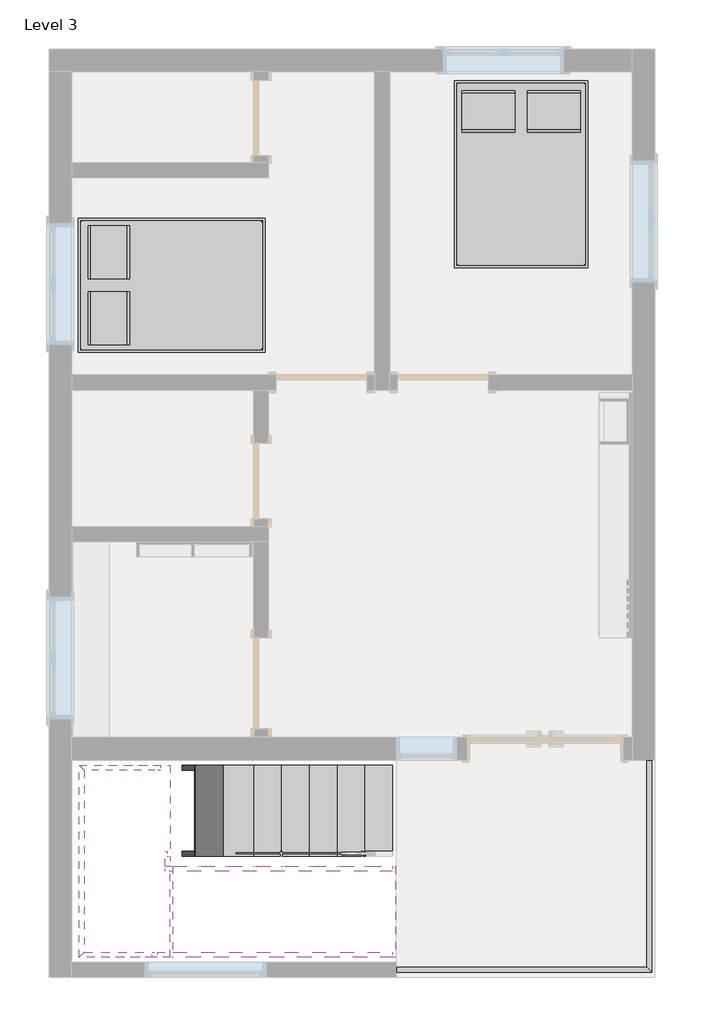
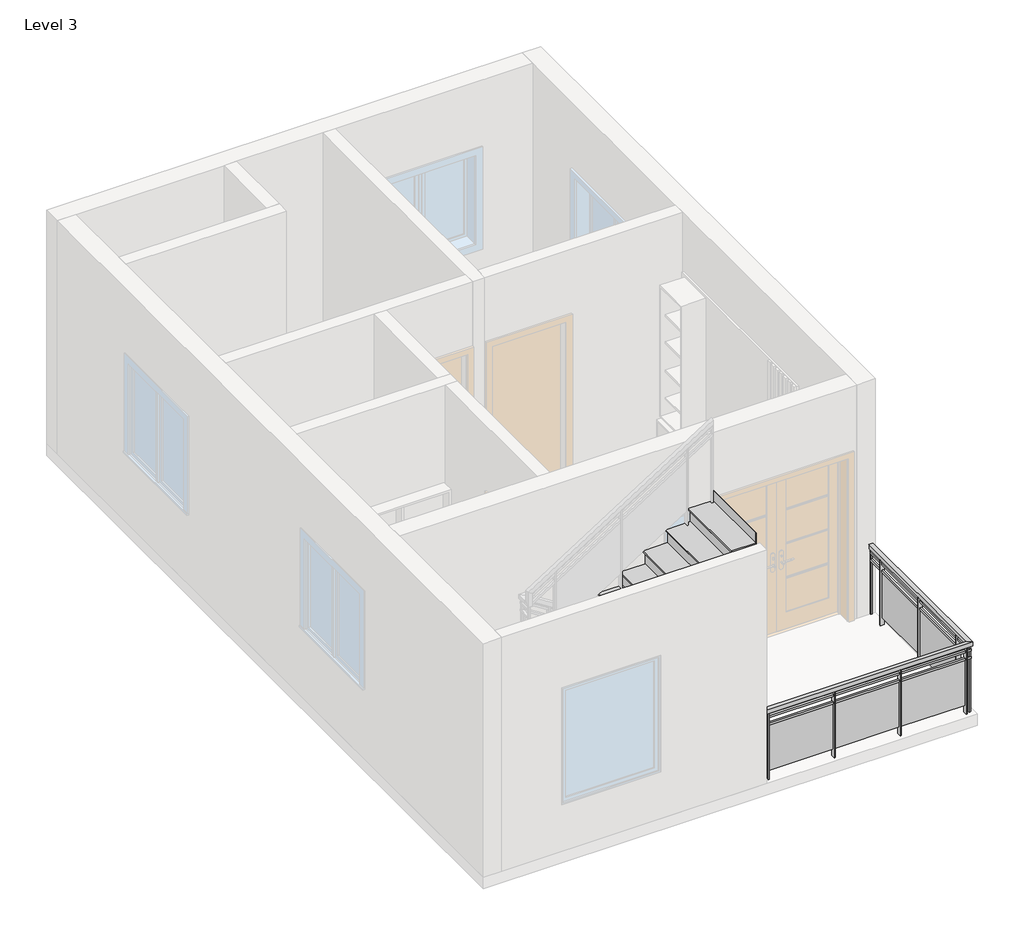
# One storey, part 2 of 2: 8 members, 2 furniture elements, 2 stair flights, 1 railing, 1 slab.
"""IFC4 building model written with IfcOpenShell, lengths in millimetres."""

from ifc_helpers import new_model, si_unit, frame, origin, place, context, project, spatial, polyline, outline, extrude, faceted_brep, transform, mapped, element, save
from components import furniture_c8abb964, non_monolithic_landing_73a33424, stair_flight_79624163, stair_flight_1f3fe34f

model = new_model("IFC4")

# Units and contexts
model_context = context("Model", 3, world=origin())
ifc_project = project(units=[si_unit("LENGTHUNIT", "METRE", prefix="MILLI")], contexts=[model_context])

# Site, building, storey
site = spatial("IfcSite", under=ifc_project)
building = spatial("IfcBuilding", under=site)
storey = spatial("IfcBuildingStorey", under=building, Name="Level 3", Elevation=6400.8)

# Furniture
placement = place(None, origin())
furniture_shape = furniture_c8abb964(model_context)
element("IfcFurniture", 1, ObjectType="Bed-Box : Double 53\" x 74\"", at=placement, inside=storey, context=model_context, shape_type="MappedRepresentation", body=[
    mapped(furniture_shape, transform((-5702.2407796, -383.210135, 6400.8), x_axis=(0.0, 0.9999999999999999, 0.0), y_axis=(-0.9999999999999999, 0.0, 0.0), z_axis=(0.0, 0.0, 1.0))),
])
element("IfcFurniture", 2, ObjectType="Bed-Box : Double 53\" x 74\"", at=placement, inside=storey, context=model_context, shape_type="MappedRepresentation", body=[
    mapped(furniture_shape, transform((-2289.0637304, 1307.9718322, 6400.8), x_axis=(1.0, 0.0, 0.0), y_axis=(0.0, 1.0, 0.0), z_axis=(0.0, 0.0, 1.0))),
])

# Members
element("IfcMember", 3, ObjectType="Carriage - 2\" Width", at=placement, inside=storey, context=model_context, shape_type="Brep", body=[
    faceted_brep([(-3245.3112714, -5936.857676, 9277.1282995), (-3245.3112714, -5886.057676, 9277.1282995), (-3245.3112714, -5886.057676, 9372.6), (-3245.3112714, -5936.857676, 9372.6), (-3492.9612714, -5886.057676, 9119.532845), (-3772.3612714, -5886.057676, 8941.732845), (-4051.7612714, -5886.057676, 8763.932845), (-4331.1612714, -5886.057676, 8586.132845), (-4610.5612714, -5886.057676, 8408.332845), (-4889.9612714, -5886.057676, 8230.532845), (-5169.3612714, -5886.057676, 8052.732845), (-5448.7612714, -5886.057676, 7874.932845), (-5480.5112714, -5886.057676, 7854.7282995), (-5531.3112714, -5886.057676, 7822.4010268), (-5531.3112714, -5886.057676, 7950.2), (-5480.5112714, -5886.057676, 7950.2), (-5448.7612714, -5886.057676, 7950.2), (-5448.7612714, -5886.057676, 8128.0), (-5169.3612714, -5886.057676, 8128.0), (-5169.3612714, -5886.057676, 8305.8), (-4889.9612714, -5886.057676, 8305.8), (-4889.9612714, -5886.057676, 8483.6), (-4610.5612714, -5886.057676, 8483.6), (-4610.5612714, -5886.057676, 8661.4), (-4331.1612714, -5886.057676, 8661.4), (-4331.1612714, -5886.057676, 8839.2), (-4051.7612714, -5886.057676, 8839.2), (-4051.7612714, -5886.057676, 9017.0), (-3772.3612714, -5886.057676, 9017.0), (-3772.3612714, -5886.057676, 9194.8), (-3492.9612714, -5886.057676, 9194.8), (-3492.9612714, -5886.057676, 9372.6), (-5531.3112714, -5936.857676, 7822.4010268), (-3492.9612714, -5936.857676, 9372.6), (-3492.9612714, -5936.857676, 9194.8), (-3772.3612714, -5936.857676, 9194.8), (-3772.3612714, -5936.857676, 9017.0), (-4051.7612714, -5936.857676, 9017.0), (-4051.7612714, -5936.857676, 8839.2), (-4331.1612714, -5936.857676, 8839.2), (-4331.1612714, -5936.857676, 8661.4), (-4610.5612714, -5936.857676, 8661.4), (-4610.5612714, -5936.857676, 8483.6), (-4889.9612714, -5936.857676, 8483.6), (-4889.9612714, -5936.857676, 8305.8), (-5169.3612714, -5936.857676, 8305.8), (-5169.3612714, -5936.857676, 8128.0), (-5448.7612714, -5936.857676, 8128.0), (-5448.7612714, -5936.857676, 7950.2), (-5531.3112714, -5936.857676, 7950.2)], [[[0, 1, 2, 3]], [[2, 1, 4, 5, 6, 7, 8, 9, 10, 11, 12, 13, 14, 15, 16, 17, 18, 19, 20, 21, 22, 23, 24, 25, 26, 27, 28, 29, 30, 31]], [[1, 0, 32, 13, 12, 11, 10, 9, 8, 7, 6, 5, 4]], [[32, 0, 3, 33, 34, 35, 36, 37, 38, 39, 40, 41, 42, 43, 44, 45, 46, 47, 48, 49]], [[17, 47, 46, 18]], [[47, 17, 16, 48]], [[19, 45, 44, 20]], [[18, 46, 45, 19]], [[21, 43, 42, 22]], [[20, 44, 43, 21]], [[23, 41, 40, 24]], [[22, 42, 41, 23]], [[25, 39, 38, 26]], [[24, 40, 39, 25]], [[27, 37, 36, 28]], [[26, 38, 37, 27]], [[29, 35, 34, 30]], [[28, 36, 35, 29]], [[31, 33, 3, 2]], [[30, 34, 33, 31]], [[13, 32, 49, 14]], [[48, 16, 15, 14, 49]]]),
])
element("IfcMember", 4, ObjectType="Carriage - 2\" Width", at=placement, inside=storey, context=model_context, shape_type="Brep", body=[
    faceted_brep([(-3245.3112714, -6800.457676, 9277.1282995), (-3245.3112714, -6749.657676, 9277.1282995), (-3245.3112714, -6749.657676, 9372.6), (-3245.3112714, -6800.457676, 9372.6), (-5609.8843135, -6749.657676, 7772.4), (-5661.6597957, -6749.657676, 7950.2), (-5448.7612714, -6749.657676, 7950.2), (-5448.7612714, -6749.657676, 8128.0), (-5169.3612714, -6749.657676, 8128.0), (-5169.3612714, -6749.657676, 8305.8), (-4889.9612714, -6749.657676, 8305.8), (-4889.9612714, -6749.657676, 8483.6), (-4610.5612714, -6749.657676, 8483.6), (-4610.5612714, -6749.657676, 8661.4), (-4331.1612714, -6749.657676, 8661.4), (-4331.1612714, -6749.657676, 8839.2), (-4051.7612714, -6749.657676, 8839.2), (-4051.7612714, -6749.657676, 9017.0), (-3772.3612714, -6749.657676, 9017.0), (-3772.3612714, -6749.657676, 9194.8), (-3492.9612714, -6749.657676, 9194.8), (-3492.9612714, -6749.657676, 9372.6), (-3492.9612714, -6800.457676, 9119.532845), (-3772.3612714, -6800.457676, 8941.732845), (-4051.7612714, -6800.457676, 8763.932845), (-4331.1612714, -6800.457676, 8586.132845), (-4610.5612714, -6800.457676, 8408.332845), (-4889.9612714, -6800.457676, 8230.532845), (-5169.3612714, -6800.457676, 8052.732845), (-5448.7612714, -6800.457676, 7874.932845), (-5480.5112714, -6800.457676, 7854.7282995), (-5609.8843135, -6800.457676, 7772.4), (-3492.9612714, -6800.457676, 9372.6), (-3492.9612714, -6800.457676, 9194.8), (-3772.3612714, -6800.457676, 9194.8), (-3772.3612714, -6800.457676, 9017.0), (-4051.7612714, -6800.457676, 9017.0), (-4051.7612714, -6800.457676, 8839.2), (-4331.1612714, -6800.457676, 8839.2), (-4331.1612714, -6800.457676, 8661.4), (-4610.5612714, -6800.457676, 8661.4), (-4610.5612714, -6800.457676, 8483.6), (-4889.9612714, -6800.457676, 8483.6), (-4889.9612714, -6800.457676, 8305.8), (-5169.3612714, -6800.457676, 8305.8), (-5169.3612714, -6800.457676, 8128.0), (-5448.7612714, -6800.457676, 8128.0), (-5448.7612714, -6800.457676, 7950.2), (-5480.5112714, -6800.457676, 7950.2), (-5661.6597957, -6800.457676, 7950.2)], [[[0, 1, 2, 3]], [[1, 4, 5, 6, 7, 8, 9, 10, 11, 12, 13, 14, 15, 16, 17, 18, 19, 20, 21, 2]], [[1, 0, 22, 23, 24, 25, 26, 27, 28, 29, 30, 31, 4]], [[0, 3, 32, 33, 34, 35, 36, 37, 38, 39, 40, 41, 42, 43, 44, 45, 46, 47, 48, 49, 31, 30, 29, 28, 27, 26, 25, 24, 23, 22]], [[7, 46, 45, 8]], [[46, 7, 6, 47]], [[9, 44, 43, 10]], [[8, 45, 44, 9]], [[11, 42, 41, 12]], [[10, 43, 42, 11]], [[13, 40, 39, 14]], [[12, 41, 40, 13]], [[15, 38, 37, 16]], [[14, 39, 38, 15]], [[17, 36, 35, 18]], [[16, 37, 36, 17]], [[19, 34, 33, 20]], [[18, 35, 34, 19]], [[21, 32, 3, 2]], [[20, 33, 32, 21]], [[4, 31, 49, 5]], [[47, 6, 5, 49, 48]]]),
])
element("IfcMember", 5, ObjectType="Carriage - 2\" Width", at=placement, inside=storey, context=model_context, shape_type="Brep", body=[
    faceted_brep([(-3277.0612714, -5784.457676, 6400.8), (-3475.1668007, -5784.457676, 6400.8), (-3475.1668007, -5733.657676, 6400.8), (-3277.0612714, -5733.657676, 6400.8), (-5480.5112714, -5784.457676, 7676.9282995), (-5480.5112714, -5733.657676, 7676.9282995), (-3556.4612714, -5784.457676, 6452.532845), (-3835.8612714, -5784.457676, 6630.332845), (-4115.2612714, -5784.457676, 6808.132845), (-4394.6612714, -5784.457676, 6985.932845), (-4674.0612714, -5784.457676, 7163.732845), (-4953.4612714, -5784.457676, 7341.532845), (-5232.8612714, -5784.457676, 7519.332845), (-5480.5112714, -5784.457676, 7772.4), (-3277.0612714, -5784.457676, 6527.8), (-3556.4612714, -5784.457676, 6527.8), (-3556.4612714, -5784.457676, 6705.6), (-3835.8612714, -5784.457676, 6705.6), (-3835.8612714, -5784.457676, 6883.4), (-4115.2612714, -5784.457676, 6883.4), (-4115.2612714, -5784.457676, 7061.2), (-4394.6612714, -5784.457676, 7061.2), (-4394.6612714, -5784.457676, 7239.0), (-4674.0612714, -5784.457676, 7239.0), (-4674.0612714, -5784.457676, 7416.8), (-4953.4612714, -5784.457676, 7416.8), (-4953.4612714, -5784.457676, 7594.6), (-5232.8612714, -5784.457676, 7594.6), (-5232.8612714, -5784.457676, 7772.4), (-5232.8612714, -5733.657676, 7772.4), (-5480.5112714, -5733.657676, 7772.4), (-5232.8612714, -5733.657676, 7594.6), (-4953.4612714, -5733.657676, 7594.6), (-4953.4612714, -5733.657676, 7416.8), (-4674.0612714, -5733.657676, 7416.8), (-4674.0612714, -5733.657676, 7239.0), (-4394.6612714, -5733.657676, 7239.0), (-4394.6612714, -5733.657676, 7061.2), (-4115.2612714, -5733.657676, 7061.2), (-4115.2612714, -5733.657676, 6883.4), (-3835.8612714, -5733.657676, 6883.4), (-3835.8612714, -5733.657676, 6705.6), (-3556.4612714, -5733.657676, 6705.6), (-3556.4612714, -5733.657676, 6527.8), (-3277.0612714, -5733.657676, 6527.8)], [[[0, 1, 2, 3]], [[4, 5, 2, 1, 6, 7, 8, 9, 10, 11, 12]], [[13, 4, 12, 11, 10, 9, 8, 7, 6, 1, 0, 14, 15, 16, 17, 18, 19, 20, 21, 22, 23, 24, 25, 26, 27, 28]], [[28, 29, 30, 13]], [[2, 5, 30, 29, 31, 32, 33, 34, 35, 36, 37, 38, 39, 40, 41, 42, 43, 44, 3]], [[44, 14, 0, 3]], [[14, 44, 43, 15]], [[15, 43, 42, 16]], [[16, 42, 41, 17]], [[17, 41, 40, 18]], [[18, 40, 39, 19]], [[19, 39, 38, 20]], [[20, 38, 37, 21]], [[21, 37, 36, 22]], [[22, 36, 35, 23]], [[23, 35, 34, 24]], [[24, 34, 33, 25]], [[25, 33, 32, 26]], [[26, 32, 31, 27]], [[27, 31, 29, 28]], [[5, 4, 13, 30]]]),
])
element("IfcMember", 6, ObjectType="Carriage - 2\" Width", at=placement, inside=storey, context=model_context, shape_type="Brep", body=[
    faceted_brep([(-3277.0612714, -4920.857676, 6400.8), (-3475.1668007, -4920.857676, 6400.8), (-3475.1668007, -4870.057676, 6400.8), (-3277.0612714, -4870.057676, 6400.8), (-5630.5382293, -4920.857676, 7772.4), (-5630.5382293, -4870.057676, 7772.4), (-5512.2612714, -4870.057676, 7697.132845), (-5480.5112714, -4870.057676, 7676.9282995), (-5232.8612714, -4870.057676, 7519.332845), (-4953.4612714, -4870.057676, 7341.532845), (-4674.0612714, -4870.057676, 7163.732845), (-4394.6612714, -4870.057676, 6985.932845), (-4115.2612714, -4870.057676, 6808.132845), (-3835.8612714, -4870.057676, 6630.332845), (-3556.4612714, -4870.057676, 6452.532845), (-5578.7627471, -4920.857676, 7950.2), (-3277.0612714, -4920.857676, 6527.8), (-3556.4612714, -4920.857676, 6527.8), (-3556.4612714, -4920.857676, 6705.6), (-3835.8612714, -4920.857676, 6705.6), (-3835.8612714, -4920.857676, 6883.4), (-4115.2612714, -4920.857676, 6883.4), (-4115.2612714, -4920.857676, 7061.2), (-4394.6612714, -4920.857676, 7061.2), (-4394.6612714, -4920.857676, 7239.0), (-4674.0612714, -4920.857676, 7239.0), (-4674.0612714, -4920.857676, 7416.8), (-4953.4612714, -4920.857676, 7416.8), (-4953.4612714, -4920.857676, 7594.6), (-5232.8612714, -4920.857676, 7594.6), (-5232.8612714, -4920.857676, 7772.4), (-5512.2612714, -4920.857676, 7772.4), (-5512.2612714, -4920.857676, 7950.2), (-5232.8612714, -4870.057676, 7772.4), (-5480.5112714, -4870.057676, 7772.4), (-5512.2612714, -4870.057676, 7772.4), (-5578.7627471, -4870.057676, 7950.2), (-5512.2612714, -4870.057676, 7950.2), (-5232.8612714, -4870.057676, 7594.6), (-4953.4612714, -4870.057676, 7594.6), (-4953.4612714, -4870.057676, 7416.8), (-4674.0612714, -4870.057676, 7416.8), (-4674.0612714, -4870.057676, 7239.0), (-4394.6612714, -4870.057676, 7239.0), (-4394.6612714, -4870.057676, 7061.2), (-4115.2612714, -4870.057676, 7061.2), (-4115.2612714, -4870.057676, 6883.4), (-3835.8612714, -4870.057676, 6883.4), (-3835.8612714, -4870.057676, 6705.6), (-3556.4612714, -4870.057676, 6705.6), (-3556.4612714, -4870.057676, 6527.8), (-3277.0612714, -4870.057676, 6527.8)], [[[0, 1, 2, 3]], [[4, 5, 6, 7, 8, 9, 10, 11, 12, 13, 14, 2, 1]], [[15, 4, 1, 0, 16, 17, 18, 19, 20, 21, 22, 23, 24, 25, 26, 27, 28, 29, 30, 31, 32]], [[30, 33, 34, 35, 31]], [[5, 36, 37, 35, 34, 33, 38, 39, 40, 41, 42, 43, 44, 45, 46, 47, 48, 49, 50, 51, 3, 2, 14, 13, 12, 11, 10, 9, 8, 7, 6]], [[51, 16, 0, 3]], [[16, 51, 50, 17]], [[17, 50, 49, 18]], [[18, 49, 48, 19]], [[19, 48, 47, 20]], [[20, 47, 46, 21]], [[21, 46, 45, 22]], [[22, 45, 44, 23]], [[23, 44, 43, 24]], [[24, 43, 42, 25]], [[25, 42, 41, 26]], [[26, 41, 40, 27]], [[27, 40, 39, 28]], [[28, 39, 38, 29]], [[29, 38, 33, 30]], [[5, 4, 15, 36]], [[31, 35, 37, 32]], [[32, 37, 36, 15]]]),
])
element("IfcMember", 7, ObjectType="Carriage - 2\" Width", at=placement, inside=storey, context=model_context, shape_type="SweptSolid", body=[
    extrude(outline(polyline([(-5531.3112714, -5886.057676), (-5531.3112714, -5733.657676), (-5512.2612714, -5733.657676), (-5512.2612714, -5784.457676), (-5480.5112714, -5784.457676), (-5480.5112714, -5886.057676), (-5531.3112714, -5886.057676)])), frame((0.0, 0.0, 7772.4), z_axis=(0.0, 0.0, 1.0), x_axis=(1.0, 0.0, 0.0)), (0.0, 0.0, 1.0), 177.8),
])
element("IfcMember", 8, ObjectType="Carriage - 2\" Width", at=placement, inside=storey, context=model_context, shape_type="Brep", body=[
    faceted_brep([(-6344.1112714, -4920.857676, 7772.4), (-5630.5382293, -4920.857676, 7772.4), (-5578.7627471, -4920.857676, 7950.2), (-6344.1112714, -4920.857676, 7950.2), (-6394.9112714, -4870.057676, 7772.4), (-5630.5382293, -4870.057676, 7772.4), (-6394.9112714, -4870.057676, 7950.2), (-5578.7627471, -4870.057676, 7950.2)], [[[0, 1, 2, 3]], [[1, 0, 4, 5]], [[5, 4, 6, 7]], [[3, 2, 7, 6]], [[1, 5, 7, 2]], [[4, 0, 3, 6]]]),
])
element("IfcMember", 9, ObjectType="Carriage - 2\" Width", at=placement, inside=storey, context=model_context, shape_type="SweptSolid", body=[
    extrude(outline(polyline([(-6344.1112714, -4920.857676), (-6344.1112714, -6749.657676), (-6394.9112714, -6800.457676), (-6394.9112714, -4870.057676), (-6344.1112714, -4920.857676)])), frame((0.0, 0.0, 7772.4), z_axis=(0.0, 0.0, 1.0), x_axis=(1.0, 0.0, 0.0)), (0.0, 0.0, 1.0), 177.8),
])
element("IfcMember", 10, ObjectType="Carriage - 2\" Width", at=placement, inside=storey, context=model_context, shape_type="Brep", body=[
    faceted_brep([(-5609.8843135, -6749.657676, 7772.4), (-6344.1112714, -6749.657676, 7772.4), (-6344.1112714, -6749.657676, 7950.2), (-5661.6597957, -6749.657676, 7950.2), (-5609.8843135, -6800.457676, 7772.4), (-6394.9112714, -6800.457676, 7772.4), (-5661.6597957, -6800.457676, 7950.2), (-6394.9112714, -6800.457676, 7950.2)], [[[0, 1, 2, 3]], [[1, 0, 4, 5]], [[5, 4, 6, 7]], [[3, 2, 7, 6]], [[1, 5, 7, 2]], [[4, 0, 3, 6]]]),
])

# Railing
element("IfcRailing", 11, ObjectType="Glass Panel - Bottom Fill", at=placement, inside=storey, context=model_context, shape_type="SolidModel", body=[
    faceted_brep([(-3198.2973712, -6902.057676, 7315.2), (-3198.2973712, -6902.057676, 7264.4), (-3198.2973712, -6952.857676, 7264.4), (-3198.2973712, -6952.857676, 7315.2), (-683.6973712, -6902.057676, 7315.2), (-683.6973712, -6902.057676, 7264.4), (-632.8973712, -6952.857676, 7264.4), (-632.8973712, -6952.857676, 7315.2), (-683.6973712, -4819.257676, 7315.2), (-632.8973712, -4819.257676, 7315.2), (-632.8973712, -4819.257676, 7264.4), (-683.6973712, -4819.257676, 7264.4)], [[[0, 1, 2, 3]], [[1, 0, 4, 5]], [[2, 1, 5, 6]], [[3, 2, 6, 7]], [[0, 3, 7, 4]], [[8, 9, 10, 11]], [[5, 4, 8, 11]], [[6, 5, 11, 10]], [[7, 6, 10, 9]], [[4, 7, 9, 8]]]),
    faceted_brep([(-3198.2973712, -6940.157676, 7226.3), (-3198.2973712, -6914.757676, 7226.3), (-3198.2973712, -6914.757676, 7200.9), (-3198.2973712, -6940.157676, 7200.9), (-645.5973712, -6940.157676, 7226.3), (-670.9973712, -6914.757676, 7226.3), (-670.9973712, -6914.757676, 7200.9), (-645.5973712, -6940.157676, 7200.9), (-645.5973712, -4819.257676, 7226.3), (-645.5973712, -4819.257676, 7200.9), (-670.9973712, -4819.257676, 7200.9), (-670.9973712, -4819.257676, 7226.3)], [[[0, 1, 2, 3]], [[1, 0, 4, 5]], [[2, 1, 5, 6]], [[3, 2, 6, 7]], [[0, 3, 7, 4]], [[8, 9, 10, 11]], [[5, 4, 8, 11]], [[6, 5, 11, 10]], [[7, 6, 10, 9]], [[4, 7, 9, 8]]]),
    faceted_brep([(-3198.2973712, -6940.157676, 7124.7), (-3198.2973712, -6914.757676, 7124.7), (-3198.2973712, -6914.757676, 7099.3), (-3198.2973712, -6940.157676, 7099.3), (-645.5973712, -6940.157676, 7124.7), (-670.9973712, -6914.757676, 7124.7), (-670.9973712, -6914.757676, 7099.3), (-645.5973712, -6940.157676, 7099.3), (-645.5973712, -4819.257676, 7124.7), (-645.5973712, -4819.257676, 7099.3), (-670.9973712, -4819.257676, 7099.3), (-670.9973712, -4819.257676, 7124.7)], [[[0, 1, 2, 3]], [[1, 0, 4, 5]], [[2, 1, 5, 6]], [[3, 2, 6, 7]], [[0, 3, 7, 4]], [[8, 9, 10, 11]], [[5, 4, 8, 11]], [[6, 5, 11, 10]], [[7, 6, 10, 9]], [[4, 7, 9, 8]]]),
    extrude(outline(polyline([(-632.8973712, -5066.907676), (-683.6973712, -5066.907676), (-683.6973712, -5054.207676), (-632.8973712, -5054.207676), (-632.8973712, -5066.907676)])), frame((0.0, 0.0, 6400.8), z_axis=(0.0, 0.0, 1.0), x_axis=(1.0, 0.0, 0.0)), (0.0, 0.0, 1.0), 863.6),
    extrude(outline(polyline([(-664.8325282, -5873.357676), (-664.8325282, -5060.557676), (-658.4825282, -5060.557676), (-658.4825282, -5873.357676), (-664.8325282, -5873.357676)])), frame((0.0, 0.0, 6502.4), z_axis=(0.0, 0.0, 1.0), x_axis=(1.0, 0.0, 0.0)), (0.0, 0.0, 1.0), 596.9),
    extrude(outline(polyline([(-632.8973712, -5879.707676), (-683.6973712, -5879.707676), (-683.6973712, -5867.007676), (-632.8973712, -5867.007676), (-632.8973712, -5879.707676)])), frame((0.0, 0.0, 6400.8), z_axis=(0.0, 0.0, 1.0), x_axis=(1.0, 0.0, 0.0)), (0.0, 0.0, 1.0), 863.6),
    extrude(outline(polyline([(-664.8325282, -6686.157676), (-664.8325282, -5873.357676), (-658.4825282, -5873.357676), (-658.4825282, -6686.157676), (-664.8325282, -6686.157676)])), frame((0.0, 0.0, 6502.4), z_axis=(0.0, 0.0, 1.0), x_axis=(1.0, 0.0, 0.0)), (0.0, 0.0, 1.0), 596.9),
    extrude(outline(polyline([(-632.8973712, -6692.507676), (-683.6973712, -6692.507676), (-683.6973712, -6679.807676), (-632.8973712, -6679.807676), (-632.8973712, -6692.507676)])), frame((0.0, 0.0, 6400.8), z_axis=(0.0, 0.0, 1.0), x_axis=(1.0, 0.0, 0.0)), (0.0, 0.0, 1.0), 863.6),
    extrude(outline(polyline([(-715.4473712, -6952.857676), (-715.4473712, -6902.057676), (-702.7473712, -6902.057676), (-702.7473712, -6952.857676), (-715.4473712, -6952.857676)])), frame((0.0, 0.0, 6400.8), z_axis=(0.0, 0.0, 1.0), x_axis=(1.0, 0.0, 0.0)), (0.0, 0.0, 1.0), 863.6),
    extrude(outline(polyline([(-1521.8973712, -6920.922519), (-709.0973712, -6920.922519), (-709.0973712, -6927.272519), (-1521.8973712, -6927.272519), (-1521.8973712, -6920.922519)])), frame((0.0, 0.0, 6502.4), z_axis=(0.0, 0.0, 1.0), x_axis=(1.0, 0.0, 0.0)), (0.0, 0.0, 1.0), 596.9),
    extrude(outline(polyline([(-1528.2473712, -6952.857676), (-1528.2473712, -6902.057676), (-1515.5473712, -6902.057676), (-1515.5473712, -6952.857676), (-1528.2473712, -6952.857676)])), frame((0.0, 0.0, 6400.8), z_axis=(0.0, 0.0, 1.0), x_axis=(1.0, 0.0, 0.0)), (0.0, 0.0, 1.0), 863.6),
    extrude(outline(polyline([(-2334.6973712, -6920.922519), (-1521.8973712, -6920.922519), (-1521.8973712, -6927.272519), (-2334.6973712, -6927.272519), (-2334.6973712, -6920.922519)])), frame((0.0, 0.0, 6502.4), z_axis=(0.0, 0.0, 1.0), x_axis=(1.0, 0.0, 0.0)), (0.0, 0.0, 1.0), 596.9),
    extrude(outline(polyline([(-2341.0473712, -6952.857676), (-2341.0473712, -6902.057676), (-2328.3473712, -6902.057676), (-2328.3473712, -6952.857676), (-2341.0473712, -6952.857676)])), frame((0.0, 0.0, 6400.8), z_axis=(0.0, 0.0, 1.0), x_axis=(1.0, 0.0, 0.0)), (0.0, 0.0, 1.0), 863.6),
    extrude(outline(polyline([(-3147.4973712, -6920.922519), (-2334.6973712, -6920.922519), (-2334.6973712, -6927.272519), (-3147.4973712, -6927.272519), (-3147.4973712, -6920.922519)])), frame((0.0, 0.0, 6502.4), z_axis=(0.0, 0.0, 1.0), x_axis=(1.0, 0.0, 0.0)), (0.0, 0.0, 1.0), 596.9),
    extrude(outline(polyline([(-3153.8473712, -6952.857676), (-3153.8473712, -6902.057676), (-3141.1473712, -6902.057676), (-3141.1473712, -6952.857676), (-3153.8473712, -6952.857676)])), frame((0.0, 0.0, 6400.8), z_axis=(0.0, 0.0, 1.0), x_axis=(1.0, 0.0, 0.0)), (0.0, 0.0, 1.0), 863.6),
    extrude(outline(polyline([(-667.8223712, -6936.982676), (-667.8223712, -6917.932676), (-648.7723712, -6917.932676), (-648.7723712, -6936.982676), (-667.8223712, -6936.982676)])), frame((0.0, 0.0, 6400.8), z_axis=(0.0, 0.0, 1.0), x_axis=(1.0, 0.0, 0.0)), (0.0, 0.0, 1.0), 863.6),
    extrude(outline(polyline([(-648.7723712, -4831.957676), (-667.8223712, -4831.957676), (-667.8223712, -4812.907676), (-648.7723712, -4812.907676), (-648.7723712, -4831.957676)])), frame((0.0, 0.0, 6400.8), z_axis=(0.0, 0.0, 1.0), x_axis=(1.0, 0.0, 0.0)), (0.0, 0.0, 1.0), 863.6),
    extrude(outline(polyline([(-3204.6473712, -6936.982676), (-3204.6473712, -6917.932676), (-3185.5973712, -6917.932676), (-3185.5973712, -6936.982676), (-3204.6473712, -6936.982676)])), frame((0.0, 0.0, 6400.8), z_axis=(0.0, 0.0, 1.0), x_axis=(1.0, 0.0, 0.0)), (0.0, 0.0, 1.0), 863.6),
])

# Slab
non_monolithic_landing_shape = non_monolithic_landing_73a33424(model_context)
element("IfcSlab", 12, ObjectType="Non-Monolithic Landing", at=placement, inside=storey, context=model_context, shape_type="MappedRepresentation", body=[
    mapped(non_monolithic_landing_shape, transform((0.0, 0.0, 0.0), x_axis=(1.0, 0.0, 0.0), y_axis=(0.0, 1.0, 0.0), z_axis=(0.0, 0.0, 1.0))),
])

# Stair flights
stair_flight_shape = stair_flight_79624163(model_context)
element("IfcStairFlight", 13, ObjectType="2\" Tread 1\" Nosing 1/4\" Riser", at=placement, inside=storey, context=model_context, shape_type="MappedRepresentation", body=[
    mapped(stair_flight_shape, transform((0.0, 0.0, 0.0), x_axis=(1.0, 0.0, 0.0), y_axis=(0.0, 1.0, 0.0), z_axis=(0.0, 0.0, 1.0))),
])
stair_flight_2_shape = stair_flight_1f3fe34f(model_context)
element("IfcStairFlight", 14, ObjectType="2\" Tread 1\" Nosing 1/4\" Riser", at=placement, inside=storey, context=model_context, shape_type="MappedRepresentation", body=[
    mapped(stair_flight_2_shape, transform((0.0, 0.0, 0.0), x_axis=(1.0, 0.0, 0.0), y_axis=(0.0, 1.0, 0.0), z_axis=(0.0, 0.0, 1.0))),
])

save(model, "model.ifc")

# Revit data of these elements
# Type "Bed-Box : Double 53\" x 74\""
#   Assembly Code = "E2020200"
#   Length = 6' - 2"
#   Width = 4' - 5"
#   Frame Material = Birch
#   Mattress Material = Linen, White
#   Default Elevation = 0
# Type "Glass Panel - Bottom Fill"
#   Assembly Code = "C2010400"
#   built-in parameter 1008612 = 0.0416667 (stored number, unit not read)
#   built-in parameter 1008611 = 0.0416667 (stored number, unit not read)
#   built-in parameter 1008609 = 0.333333 (stored number, unit not read)
#   built-in parameter 1008604 = 0.166667 (stored number, unit not read)
#   built-in parameter 1008603 = 0.166667 (stored number, unit not read)
#   Railing Height = 3' - 0"
#   built-in parameter 1008630 = 2
#   built-in parameter 1008610 = 2
#   built-in parameter 1008618 = Baluster - Square : 3/4"
# Elements 1, 2 (IfcFurniture, "Bed-Box : Double 53\" x 74\"")
#   Phase Created = New Construction
#   Materials on its faces: "Birch", "Linen, White"
# Elements 3, 4, 5, 6, 7, 8, 9, 10 (IfcMember, "Carriage - 2\" Width")
#   Phase Created = New Construction
# Element 11 (IfcRailing, "Glass Panel - Bottom Fill")
#   Phase Created = New Construction
#   Materials on its faces: "Glass"
# Element 12 (IfcSlab, "Non-Monolithic Landing")
#   Phase Created = New Construction
# Elements 13, 14 (IfcStairFlight, "2\" Tread 1\" Nosing 1/4\" Riser")
#   Phase Created = New Construction
# Materials
#   "Birch": class "Wood", colour RGB 224 178 126, transparency 0, Description = "Betula Alleghaniensis", Cost = 0
#   "Linen, White": class "Textile", colour RGB 247 247 239, transparency 0, Description = "Linen, white", Cost = 0
#   "Glass": class "Glass", colour RGB 0 128 192, transparency 0.75, Description = "Soda Lime Glass", Cost = 0
